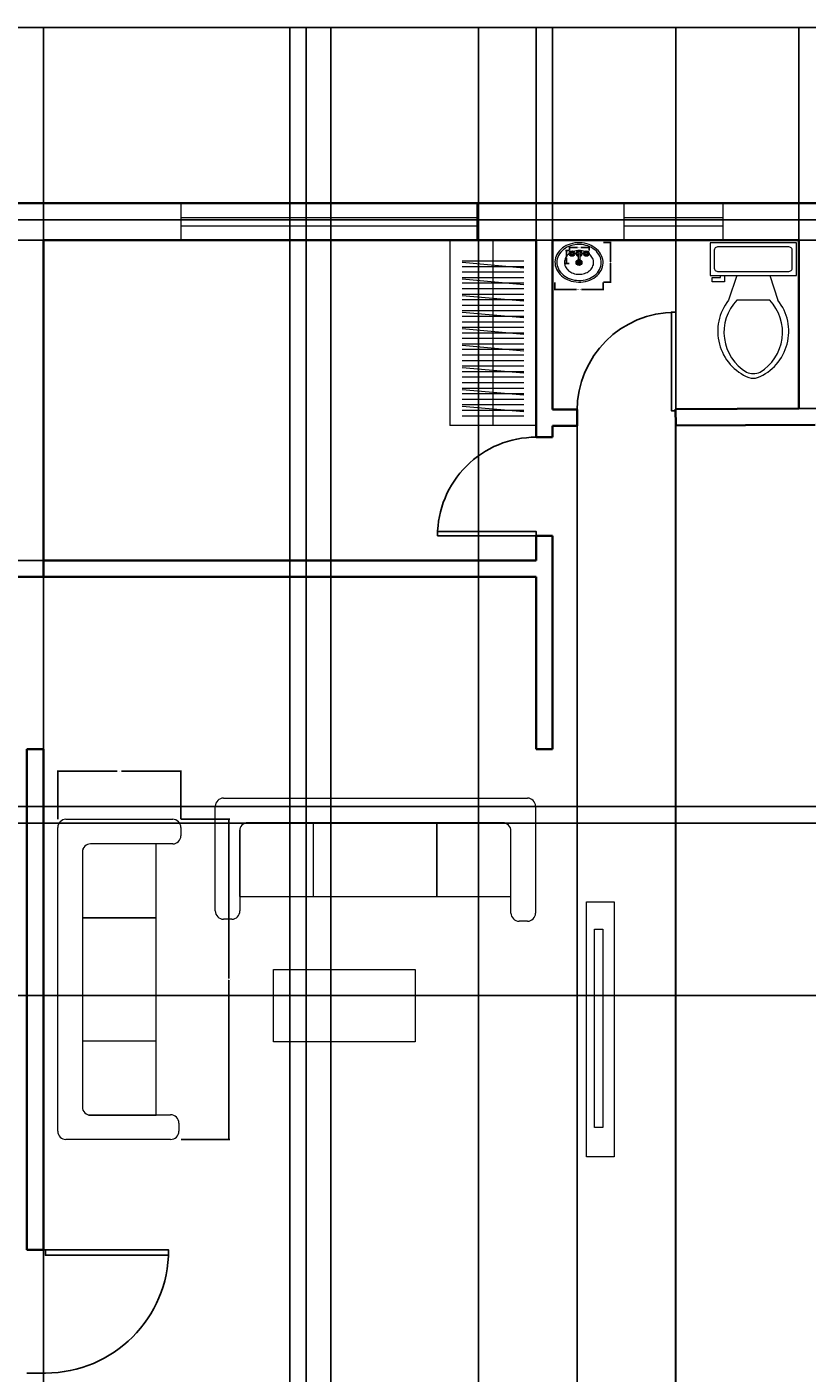
# Model space of a CAD drawing. Units: inches. Extents: x 2024 to 2965, y 1692 to 2308.
# Tile 6 of 8: x 2355 to 2545, y 1980 to 2308. Entities that reach past the tile are written whole.
import ezdxf

# ---------------------------------------------------------------- set-up
doc = ezdxf.new("R2010")
doc.units = ezdxf.units.IN
for name, color, linetype, lineweight in [('A-ANNO-DIMS', 2, 'Continuous', 18), ('A-DOOR', 3, 'Continuous', 25), ('A-EQPM', 6, 'Continuous', 18), ('A-FLOR-CASE', 33, 'Continuous', 20), ('A-FLOR-CASE-PATT', 252, 'Continuous', 13), ('A-FLOR-FIXT', 9, 'Continuous', 18), ('A-FURN', 8, 'Continuous', 18), ('A-GLAZ', 4, 'Continuous', 18), ('A-WALL', 7, 'Continuous', 35)]:
    doc.layers.add(name, color=color, linetype=linetype, lineweight=lineweight)
doc.styles.get("Standard").update_dxf_attribs({"font": 'arial.ttf'})
doc.dimstyles.get("Standard").update_dxf_attribs({"dimtxt": 0.18, "dimasz": 0.18, "dimexe": 0.18, "dimexo": 0.0625, "dimgap": 0.09, "dimtad": 0, "dimtih": 1, "dimtoh": 1, "dimdec": 4, "dimzin": 0, "dimdsep": 46, "dimtxsty": 'Standard', "dimcen": 0.09, "dimadec": 0, "dimazin": 0, "dimtfac": 1, "dimtdec": 4, "dimtofl": 0, "dimtmove": 0, "dimatfit": 3, "dimfxl": 1, "dimtolj": 1, "dimtzin": 0, "dimarcsym": 0})

# ---------------------------------------------------------------- blocks, each defined once
blk = doc.blocks.new('*U7')
for p, q in [((0, 0), (0, -6)), ((40, 0), (40, -6))]:
    blk.add_line(p, q)
blk.add_lwpolyline([(0, 0), (0, 40), (1.75, 40), (1.75, 0)], close=True)
blk.add_arc((0, 0), 40, 0, 90)
blk = doc.blocks.new('*U6')
for p, q in [((0, 0), (0, 6)), ((40, 0), (40, 6))]:
    blk.add_line(p, q)
blk.add_lwpolyline([(0, 0), (0, -40), (1.75, -40), (1.75, 0)], close=True)
blk.add_arc((0, 0), 40, 270, 0)
blk = doc.blocks.new('Sink - Oval top')
for p, q in [((-1, 0), (1, 0)), ((0, 1), (0, -1))]:
    blk.add_line(p, q)
for points in [[(-12.23, 0.39, 0.117634), (-11.46, -3.36, 0.104469), (-8.88, -6.8, 0.090016), (-5.08, -9.07, 0.08192), (-0.32, -10.02, 0.08192), (4.49, -9.38, 0.090016), (8.42, -7.36, 0.104469), (11.22, -4.09, 0.117634), (12.23, -0.39, 0.117634), (11.46, 3.36, 0.104469), (8.88, 6.8, 0.090016), (5.08, 9.07, 0.08192), (0.32, 10.02, 0.08192), (-4.49, 9.38, 0.090016), (-8.42, 7.36, 0.104469), (-11.22, 4.09, 0.117634)], [(-11.29, 0.16, 0.118622), (-10.52, -3.25, 0.104678), (-8.07, -6.36, 0.089562), (-4.54, -8.37, 0.081185), (-0.13, -9.15, 0.081185), (4.3, -8.49, 0.089562), (7.89, -6.58, 0.104678), (10.42, -3.55, 0.118622), (11.29, -0.16, 0.118622), (10.52, 3.25, 0.104678), (8.07, 6.36, 0.089562), (4.54, 8.37, 0.081185), (0.13, 9.15, 0.081185), (-4.3, 8.49, 0.089562), (-7.89, 6.58, 0.104678), (-10.42, 3.55, 0.118622)], [(-7.42, 0.08, 0.118283), (-6.91, -2.17, 0.104607), (-5.29, -4.21, 0.089718), (-2.97, -5.53, 0.081436), (-0.07, -6.04, 0.081436), (2.84, -5.59, 0.089718), (5.2, -4.33, 0.104607), (6.86, -2.32, 0.118283), (7.42, -0.08, 0.118283), (6.91, 2.17, 0.104607), (5.29, 4.21, 0.089718), (2.97, 5.53, 0.081436), (0.07, 6.04, 0.081436), (-2.84, 5.59, 0.089718), (-5.2, 4.33, 0.104607), (-6.86, 2.32, 0.118283)]]:
    blk.add_lwpolyline(points, format="xyb", close=True)
for radius in [1.5, 1]:
    blk.add_circle((0, 0), radius)
blk = doc.blocks.new('Faucet - Bathroom top')
for p, q in [((-4.107, 0.125), (-4.375, 0.125)), ((-3.75, 0.4788), (-3.75, 0.75)), ((-3.5, 0.482), (-3.5, 0.75)), ((-3.1461, 0.125), (-2.875, 0.125)), ((3.143, 0.125), (2.875, 0.125)), ((3.5, 0.4788), (3.5, 0.75)), ((3.75, 0.482), (3.75, 0.75)), ((4.1039, 0.125), (4.375, 0.125)), ((-4.1039, -0.125), (-4.375, -0.125)), ((-3.75, -0.4821), (-3.75, -0.75)), ((-3.5, -0.4789), (-3.5, -0.75)), ((-3.143, -0.125), (-2.875, -0.125)), ((-0.5, -0.8639), (-0.5, -4.5)), ((0.5, -4.5), (0.5, -0.8631)), ((3.1461, -0.125), (2.875, -0.125)), ((3.5, -0.4821), (3.5, -0.75)), ((3.75, -0.4789), (3.75, -0.75)), ((4.107, -0.125), (4.375, -0.125))]:
    blk.add_line(p, q)
for centre, radius in [((-3.625, 0), 1.375), ((-4.625, 0), 0.2795), ((-3.625, 0), 0.5), ((-3.625, 1), 0.2795), ((-2.625, 0), 0.2795), ((0, 0), 0.5), ((3.625, 0), 1.375), ((2.625, 0), 0.2795), ((3.625, 0), 0.5), ((3.625, 1), 0.2795), ((4.625, 0), 0.2795), ((-3.625, -1), 0.2795), ((3.625, -1), 0.2795)]:
    blk.add_circle(centre, radius)
for centre, radius, start, end in [((-3.625, 0), 1, 105.2407, 164.2093), ((-3.625, 0), 1, 16.44125, 74.07887), ((0, 0), 1.5, 289.6514, 250.3603), ((0, 0), 1, 300.3431, 239.7554), ((3.625, 0), 1, 106.12, 164.0884), ((3.625, 0), 1, 16.23422, 73.90469), ((-3.625, 0), 1, 196.2342, 253.9047), ((-3.625, 0), 1, 286.12, 344.0884), ((0, -4.5), 0.5, 180, 0), ((3.625, 0), 1, 196.4413, 254.0789), ((3.625, 0), 1, 285.2407, 344.2093)]:
    blk.add_arc(centre, radius, start, end)
blk = doc.blocks.new('Toilet - top')
for p, q in [((9.5, -6), (9.5, -2)), ((-10, -8.5), (-8, -8.5)), ((-10, -9.5), (-10, -8.5)), ((-7, -9.5), (-10, -9.5)), ((-8, -8.5), (-8, -8)), ((-7, -8), (-7, -9.5)), ((-4, -8), (-6, -14)), ((4, -8), (6, -14)), ((4, -14), (-4, -14))]:
    blk.add_line(p, q)
blk.add_lwpolyline([(10.5, -8), (10.5, 0), (-10.5, 0), (-10.5, -8)], close=True)
for points in [[(-9.5, -2), (-9.5, -6)], [(8.5, -1), (-8.5, -1)], [(-8.5, -7), (8.5, -7)]]:
    blk.add_lwpolyline(points)
for centre, radius, start, end in [((-8.62, -1.88), 0.884, 81.8699, 188.1301), ((8.62, -1.88), 0.884, 351.8699, 98.1301), ((-8.62, -6.12), 0.884, 171.8699, 278.1301), ((8.62, -6.12), 0.884, 261.8699, 8.1301), ((3.52, -21.58), 12.17, 141.4691, 247.9714), ((4.2, -21.82), 11.33, 136.3677, 238.9468), ((-3.52, -21.58), 12.17, 292.0284, 38.5307), ((-4.2, -21.82), 11.33, 301.053, 43.6321), ((0, -27.88), 4, 245.7318, 294.2682), ((0, -29), 4, 254.8605, 285.1395)]:
    blk.add_arc(centre, radius, start, end)
blk = doc.blocks.new('WIN-24-D9')
for p, q in [((0, 5.5), (24, 5.5)), ((0, 3.5), (24, 3.5))]:
    blk.add_line(p, q)
for points in [[(0, 0), (0, 9)], [(24, 9), (24, 0)]]:
    blk.add_lwpolyline(points)
blk = doc.blocks.new('WIN-72-D9')
for p, q in [((0, 5.5), (72, 5.5)), ((0, 3.5), (72, 3.5))]:
    blk.add_line(p, q)
for points in [[(0, 0), (0, 9)], [(72, 9), (72, 0)]]:
    blk.add_lwpolyline(points)
blk = doc.blocks.new('SOFA-78')
for p, q in [((2, 30), (76, 30)), ((0, 2.5), (0, 28)), ((78, 28), (78, 2)), ((70, 24), (7.91, 24)), ((6, 22.6), (6, 2.5)), ((72, 2), (72, 22)), ((4, 0.5), (2, 0.5)), ((76, 0), (74, 0))]:
    blk.add_line(p, q)
for points in [[(23.94, 24), (7.91, 24, 0.414214), (5.91, 22), (5.91, 6.04), (23.94, 6.04)], [(70, 24), (53.97, 24), (53.97, 6.04), (72, 6.04), (72, 22, 0.414214)]]:
    blk.add_lwpolyline(points, format="xyb", close=True)
for points in [[(35.94, 24), (17.9, 24)], [(35.94, 6.04), (53.97, 6.04), (53.97, 24), (35.94, 24)], [(17.9, 6.04), (35.94, 6.04)]]:
    blk.add_lwpolyline(points)
for centre, start, end in [((2, 28), 90, 180), ((76, 28), 0, 90), ((70, 22), 0, 90), ((2, 2.5), 180, 270), ((4, 2.5), 270, 0), ((74, 2), 180, 270), ((76, 2), 270, 0)]:
    blk.add_arc(centre, 2, start, end)
blk = doc.blocks.new('COFFEE-TABLE')
blk.add_lwpolyline([(0, 17.56), (34.53, 17.56), (34.53, 0), (0, 0)], close=True)
blk = doc.blocks.new('*D39')
at = {"layer": 'A-ANNO-DIMS', "color": 0, "lineweight": -2, "transparency": 16777216}
for p, q in [((2392.47, 2114.69), (2404.29, 2114.69)), ((2404.11, 2114.51), (2404.11, 2075.87)), ((2404.11, 2036.87), (2404.11, 2075.5)), ((2392.47, 2036.69), (2404.29, 2036.69))]:
    blk.add_line(p, q, dxfattribs=at)
at = {"layer": 'A-ANNO-DIMS', "color": 0, "transparency": 16777216}
for points in [[(2404.08, 2114.51), (2404.14, 2114.51), (2404.11, 2114.69)], [(2404.08, 2036.87), (2404.14, 2036.87), (2404.11, 2036.69)]]:
    blk.add_solid(points, dxfattribs=at)
at = {"layer": 'Defpoints', "color": 0, "transparency": 16777216}
for p in [(2392.41, 2114.69), (2404.11, 2114.69), (2392.41, 2036.69)]:
    blk.add_point(p, dxfattribs=at)
at = {"layer": 'A-ANNO-DIMS', "color": 0, "transparency": 16777216, "insert": (2404.11, 2075.69), "char_height": 0.18, "attachment_point": 5}
blk.add_mtext('\\A1;SOFA 78 TYP.', dxfattribs=at)
blk = doc.blocks.new('*D40')
at = {"layer": 'A-ANNO-DIMS', "color": 0, "lineweight": -2, "transparency": 16777216}
for p, q in [((2362.41, 2114.75), (2362.41, 2126.57)), ((2362.59, 2126.39), (2376.88, 2126.39)), ((2392.23, 2126.39), (2377.93, 2126.39)), ((2392.41, 2114.75), (2392.41, 2126.57))]:
    blk.add_line(p, q, dxfattribs=at)
at = {"layer": 'A-ANNO-DIMS', "color": 0, "transparency": 16777216}
for points in [[(2362.59, 2126.42), (2362.59, 2126.36), (2362.41, 2126.39)], [(2392.23, 2126.42), (2392.23, 2126.36), (2392.41, 2126.39)]]:
    blk.add_solid(points, dxfattribs=at)
at = {"layer": 'Defpoints', "color": 0, "transparency": 16777216}
for p in [(2362.41, 2126.39), (2362.41, 2114.69), (2392.41, 2114.69)]:
    blk.add_point(p, dxfattribs=at)
at = {"layer": 'A-ANNO-DIMS', "color": 0, "transparency": 16777216, "insert": (2377.41, 2126.39), "char_height": 0.18, "attachment_point": 5}
blk.add_mtext('\\A1;30 TYP.', dxfattribs=at)
blk = doc.blocks.new('*D61')
at = {"layer": 'A-ANNO-DIMS', "color": 0, "lineweight": -2, "transparency": 16777216}
for p, q in [((2483.49, 2245.46), (2483.49, 2243.58)), ((2483.67, 2243.76), (2488.74, 2243.76)), ((2495.07, 2243.76), (2490, 2243.76)), ((2495.25, 2245.46), (2495.25, 2243.58))]:
    blk.add_line(p, q, dxfattribs=at)
at = {"layer": 'A-ANNO-DIMS', "color": 0, "transparency": 16777216}
for points in [[(2483.67, 2243.79), (2483.67, 2243.73), (2483.49, 2243.76)], [(2495.07, 2243.79), (2495.07, 2243.73), (2495.25, 2243.76)]]:
    blk.add_solid(points, dxfattribs=at)
at = {"layer": 'Defpoints', "color": 0, "transparency": 16777216}
for p in [(2483.49, 2245.52), (2495.25, 2245.52), (2495.25, 2243.76)]:
    blk.add_point(p, dxfattribs=at)
at = {"layer": 'A-ANNO-DIMS', "color": 0, "transparency": 16777216, "insert": (2489.37, 2243.76), "char_height": 0.18, "attachment_point": 5}
blk.add_mtext('\\A1;BASIN 12', dxfattribs=at)
blk = doc.blocks.new('*D62')
at = {"layer": 'A-ANNO-DIMS', "color": 0, "lineweight": -2, "transparency": 16777216}
for p, q in [((2495.31, 2255.17), (2497.19, 2255.17)), ((2497.01, 2254.99), (2497.01, 2250.53)), ((2497.01, 2245.7), (2497.01, 2250.17)), ((2495.31, 2245.52), (2497.19, 2245.52))]:
    blk.add_line(p, q, dxfattribs=at)
at = {"layer": 'A-ANNO-DIMS', "color": 0, "transparency": 16777216}
for points in [[(2496.98, 2254.99), (2497.04, 2254.99), (2497.01, 2255.17)], [(2496.98, 2245.7), (2497.04, 2245.7), (2497.01, 2245.52)]]:
    blk.add_solid(points, dxfattribs=at)
at = {"layer": 'Defpoints', "color": 0, "transparency": 16777216}
for p in [(2495.25, 2255.17), (2497.01, 2255.17), (2495.25, 2245.52)]:
    blk.add_point(p, dxfattribs=at)
at = {"layer": 'A-ANNO-DIMS', "color": 0, "transparency": 16777216, "insert": (2497.01, 2250.35), "char_height": 0.18, "attachment_point": 5}
blk.add_mtext('\\A1;10', dxfattribs=at)
blk = doc.blocks.new('*D67')
at = {"layer": 'A-ANNO-DIMS', "color": 0, "lineweight": -2, "transparency": 16777216}
for p, q in [((2487.01, 2253.3), (2487.01, 2254.14)), ((2487.19, 2253.96), (2488.97, 2253.96)), ((2491.62, 2253.96), (2489.83, 2253.96)), ((2491.8, 2253.3), (2491.8, 2254.14))]:
    blk.add_line(p, q, dxfattribs=at)
at = {"layer": 'A-ANNO-DIMS', "color": 0, "transparency": 16777216}
for points in [[(2487.19, 2253.99), (2487.19, 2253.93), (2487.01, 2253.96)], [(2491.62, 2253.99), (2491.62, 2253.93), (2491.8, 2253.96)]]:
    blk.add_solid(points, dxfattribs=at)
at = {"layer": 'Defpoints', "color": 0, "transparency": 16777216}
for p in [(2487.01, 2253.24), (2491.8, 2253.96), (2491.8, 2253.24)]:
    blk.add_point(p, dxfattribs=at)
at = {"layer": 'A-ANNO-DIMS', "color": 0, "transparency": 16777216, "insert": (2489.4, 2253.96), "char_height": 0.18, "attachment_point": 5}
blk.add_mtext('\\A1;TAP 5', dxfattribs=at)
blk = doc.blocks.new('*D68')
at = {"layer": 'A-ANNO-DIMS', "color": 0, "lineweight": -2, "transparency": 16777216}
for p, q in [((2486.94, 2253.24), (2486.11, 2253.24)), ((2486.29, 2253.06), (2486.29, 2251.86)), ((2486.94, 2250.13), (2486.11, 2250.13)), ((2486.29, 2250.31), (2486.29, 2251.5))]:
    blk.add_line(p, q, dxfattribs=at)
at = {"layer": 'A-ANNO-DIMS', "color": 0, "transparency": 16777216}
for points in [[(2486.26, 2253.06), (2486.32, 2253.06), (2486.29, 2253.24)], [(2486.26, 2250.31), (2486.32, 2250.31), (2486.29, 2250.13)]]:
    blk.add_solid(points, dxfattribs=at)
at = {"layer": 'Defpoints', "color": 0, "transparency": 16777216}
for p in [(2486.29, 2253.24), (2487.01, 2253.24), (2487.01, 2250.13)]:
    blk.add_point(p, dxfattribs=at)
at = {"layer": 'A-ANNO-DIMS', "color": 0, "transparency": 16777216, "insert": (2486.29, 2251.68), "char_height": 0.18, "attachment_point": 5}
blk.add_mtext('\\A1;3', dxfattribs=at)
blk = doc.blocks.new('*D76')
at = {"layer": 'A-ANNO-DIMS', "color": 0, "lineweight": -2, "transparency": 16777216}
for p, q in [((2718.97, 2264.77), (2964.97, 2264.77)), ((2964.79, 2264.59), (2964.79, 2000.12)), ((2964.79, 1735.28), (2964.79, 1999.75)), ((2515.28, 1735.1), (2964.97, 1735.1))]:
    blk.add_line(p, q, dxfattribs=at)
at = {"layer": 'A-ANNO-DIMS', "color": 0, "transparency": 16777216}
for points in [[(2964.76, 2264.59), (2964.82, 2264.59), (2964.79, 2264.77)], [(2964.76, 1735.28), (2964.82, 1735.28), (2964.79, 1735.1)]]:
    blk.add_solid(points, dxfattribs=at)
at = {"layer": 'Defpoints', "color": 0, "transparency": 16777216}
for p in [(2718.91, 2264.77), (2515.22, 1735.1), (2964.79, 1735.1)]:
    blk.add_point(p, dxfattribs=at)
at = {"layer": 'A-ANNO-DIMS', "color": 0, "transparency": 16777216, "insert": (2964.79, 1999.94), "char_height": 0.18, "attachment_point": 5}
blk.add_mtext('\\A1;529.7', dxfattribs=at)
blk = doc.blocks.new('*D80')
at = {"layer": 'A-ANNO-DIMS', "color": 0, "lineweight": -2, "transparency": 16777216}
for p, q in [((2358.91, 2255.84), (2358.91, 2307.73)), ((2359.09, 2307.55), (2418.63, 2307.55)), ((2478.73, 2307.55), (2419.19, 2307.55)), ((2478.91, 2255.84), (2478.91, 2307.73))]:
    blk.add_line(p, q, dxfattribs=at)
at = {"layer": 'A-ANNO-DIMS', "color": 0, "transparency": 16777216}
for points in [[(2359.09, 2307.58), (2359.09, 2307.52), (2358.91, 2307.55)], [(2478.73, 2307.58), (2478.73, 2307.52), (2478.91, 2307.55)]]:
    blk.add_solid(points, dxfattribs=at)
at = {"layer": 'Defpoints', "color": 0, "transparency": 16777216}
for p in [(2478.91, 2307.55), (2358.91, 2255.77), (2478.91, 2255.77)]:
    blk.add_point(p, dxfattribs=at)
at = {"layer": 'A-ANNO-DIMS', "color": 0, "transparency": 16777216, "insert": (2418.91, 2307.55), "char_height": 0.18, "attachment_point": 5}
blk.add_mtext('\\A1;120', dxfattribs=at)
blk = doc.blocks.new('*D81')
at = {"layer": 'A-ANNO-DIMS', "color": 0, "lineweight": -2, "transparency": 16777216}
for p, q in [((2478.84, 2255.77), (2024.5, 2255.77)), ((2024.68, 2255.59), (2024.68, 2216.96)), ((2024.68, 2177.95), (2024.68, 2216.59)), ((2478.84, 2177.77), (2024.5, 2177.77))]:
    blk.add_line(p, q, dxfattribs=at)
at = {"layer": 'A-ANNO-DIMS', "color": 0, "transparency": 16777216}
for points in [[(2024.65, 2255.59), (2024.71, 2255.59), (2024.68, 2255.77)], [(2024.65, 2177.95), (2024.71, 2177.95), (2024.68, 2177.77)]]:
    blk.add_solid(points, dxfattribs=at)
at = {"layer": 'Defpoints', "color": 0, "transparency": 16777216}
for p in [(2478.91, 2255.77), (2024.68, 2177.77), (2478.91, 2177.77)]:
    blk.add_point(p, dxfattribs=at)
at = {"layer": 'A-ANNO-DIMS', "color": 0, "transparency": 16777216, "insert": (2024.68, 2216.77), "char_height": 0.18, "attachment_point": 5}
blk.add_mtext('\\A1;78', dxfattribs=at)
blk = doc.blocks.new('*D84')
at = {"layer": 'A-ANNO-DIMS', "color": 0, "lineweight": -2, "transparency": 16777216}
for p, q in [((2618.84, 2255.77), (2024.5, 2255.77)), ((2024.68, 2255.59), (2024.68, 2163.96)), ((2024.68, 2071.95), (2024.68, 2163.59)), ((2618.84, 2071.77), (2024.5, 2071.77))]:
    blk.add_line(p, q, dxfattribs=at)
at = {"layer": 'A-ANNO-DIMS', "color": 0, "transparency": 16777216}
for points in [[(2024.65, 2255.59), (2024.71, 2255.59), (2024.68, 2255.77)], [(2024.65, 2071.95), (2024.71, 2071.95), (2024.68, 2071.77)]]:
    blk.add_solid(points, dxfattribs=at)
at = {"layer": 'Defpoints', "color": 0, "transparency": 16777216}
for p in [(2024.68, 2255.77), (2618.91, 2255.77), (2618.91, 2071.77)]:
    blk.add_point(p, dxfattribs=at)
at = {"layer": 'A-ANNO-DIMS', "color": 0, "transparency": 16777216, "insert": (2024.68, 2163.77), "char_height": 0.18, "attachment_point": 5}
blk.add_mtext('\\A1;184', dxfattribs=at)
blk = doc.blocks.new('*D88')
at = {"layer": 'A-ANNO-DIMS', "color": 0, "lineweight": -2, "transparency": 16777216}
for p, q in [((2817.84, 2260.77), (2024.5, 2260.77)), ((2024.68, 2260.59), (2024.68, 2189.46)), ((2024.68, 2117.95), (2024.68, 2189.09)), ((2817.84, 2117.77), (2024.5, 2117.77))]:
    blk.add_line(p, q, dxfattribs=at)
at = {"layer": 'A-ANNO-DIMS', "color": 0, "transparency": 16777216}
for points in [[(2024.65, 2260.59), (2024.71, 2260.59), (2024.68, 2260.77)], [(2024.65, 2117.95), (2024.71, 2117.95), (2024.68, 2117.77)]]:
    blk.add_solid(points, dxfattribs=at)
at = {"layer": 'Defpoints', "color": 0, "transparency": 16777216}
for p in [(2817.91, 2260.77), (2024.68, 2117.77), (2817.91, 2117.77)]:
    blk.add_point(p, dxfattribs=at)
at = {"layer": 'A-ANNO-DIMS', "color": 0, "transparency": 16777216, "insert": (2024.68, 2189.27), "char_height": 0.18, "attachment_point": 5}
blk.add_mtext('\\A1;143', dxfattribs=at)
blk = doc.blocks.new('*D93')
at = {"layer": 'A-ANNO-DIMS', "color": 0, "lineweight": -2, "transparency": 16777216}
for p, q in [((2187.46, 1932.41), (2187.46, 2307.73)), ((2187.64, 2307.55), (2302.72, 2307.55)), ((2418.73, 2307.55), (2303.65, 2307.55)), ((2418.91, 1933.84), (2418.91, 2307.73))]:
    blk.add_line(p, q, dxfattribs=at)
at = {"layer": 'A-ANNO-DIMS', "color": 0, "transparency": 16777216}
for points in [[(2187.64, 2307.58), (2187.64, 2307.52), (2187.46, 2307.55)], [(2418.73, 2307.58), (2418.73, 2307.52), (2418.91, 2307.55)]]:
    blk.add_solid(points, dxfattribs=at)
at = {"layer": 'Defpoints', "color": 0, "transparency": 16777216}
for p in [(2418.91, 2307.55), (2187.46, 1932.35), (2418.91, 1933.77)]:
    blk.add_point(p, dxfattribs=at)
at = {"layer": 'A-ANNO-DIMS', "color": 0, "transparency": 16777216, "insert": (2303.18, 2307.55), "char_height": 0.18, "attachment_point": 5}
blk.add_mtext('\\A1;231.45', dxfattribs=at)
blk = doc.blocks.new('*D96')
at = {"layer": 'A-ANNO-DIMS', "color": 0, "lineweight": -2, "transparency": 16777216}
for p, q in [((2358.91, 1889.84), (2358.91, 2307.73)), ((2359.09, 2307.55), (2388.69, 2307.55)), ((2418.73, 2307.55), (2389.13, 2307.55)), ((2418.91, 1889.84), (2418.91, 2307.73))]:
    blk.add_line(p, q, dxfattribs=at)
at = {"layer": 'A-ANNO-DIMS', "color": 0, "transparency": 16777216}
for points in [[(2359.09, 2307.58), (2359.09, 2307.52), (2358.91, 2307.55)], [(2418.73, 2307.58), (2418.73, 2307.52), (2418.91, 2307.55)]]:
    blk.add_solid(points, dxfattribs=at)
at = {"layer": 'Defpoints', "color": 0, "transparency": 16777216}
for p in [(2418.91, 2307.55), (2358.91, 1889.77), (2418.91, 1889.77)]:
    blk.add_point(p, dxfattribs=at)
at = {"layer": 'A-ANNO-DIMS', "color": 0, "transparency": 16777216, "insert": (2388.91, 2307.55), "char_height": 0.18, "attachment_point": 5}
blk.add_mtext('\\A1;60', dxfattribs=at)
blk = doc.blocks.new('*D98')
at = {"layer": 'A-ANNO-DIMS', "color": 0, "lineweight": -2, "transparency": 16777216}
for p, q in [((2422.91, 1973.84), (2422.91, 2307.73)), ((2423.09, 2307.55), (2543.62, 2307.55)), ((2664.73, 2307.55), (2544.2, 2307.55)), ((2664.91, 1956.85), (2664.91, 2307.73))]:
    blk.add_line(p, q, dxfattribs=at)
at = {"layer": 'A-ANNO-DIMS', "color": 0, "transparency": 16777216}
for points in [[(2423.09, 2307.58), (2423.09, 2307.52), (2422.91, 2307.55)], [(2664.73, 2307.58), (2664.73, 2307.52), (2664.91, 2307.55)]]:
    blk.add_solid(points, dxfattribs=at)
at = {"layer": 'Defpoints', "color": 0, "transparency": 16777216}
for p in [(2664.91, 2307.55), (2422.91, 1973.77), (2664.91, 1956.79)]:
    blk.add_point(p, dxfattribs=at)
at = {"layer": 'A-ANNO-DIMS', "color": 0, "transparency": 16777216, "insert": (2543.91, 2307.55), "char_height": 0.18, "attachment_point": 5}
blk.add_mtext('\\A1;242', dxfattribs=at)
blk = doc.blocks.new('*D101')
at = {"layer": 'A-ANNO-DIMS', "color": 0, "lineweight": -2, "transparency": 16777216}
for p, q in [((2917.96, 2113.77), (2024.5, 2113.77)), ((2024.68, 2113.59), (2024.68, 2035.52)), ((2024.68, 1957.09), (2024.68, 2035.16)), ((2917.96, 1956.91), (2024.5, 1956.91))]:
    blk.add_line(p, q, dxfattribs=at)
at = {"layer": 'A-ANNO-DIMS', "color": 0, "transparency": 16777216}
for points in [[(2024.65, 2113.59), (2024.71, 2113.59), (2024.68, 2113.77)], [(2024.65, 1957.09), (2024.71, 1957.09), (2024.68, 1956.91)]]:
    blk.add_solid(points, dxfattribs=at)
at = {"layer": 'Defpoints', "color": 0, "transparency": 16777216}
for p in [(2024.68, 2113.77), (2918.02, 2113.77), (2918.02, 1956.91)]:
    blk.add_point(p, dxfattribs=at)
at = {"layer": 'A-ANNO-DIMS', "color": 0, "transparency": 16777216, "insert": (2024.68, 2035.34), "char_height": 0.18, "attachment_point": 5}
blk.add_mtext('\\A1;156.87', dxfattribs=at)
blk = doc.blocks.new('*D103')
at = {"layer": 'A-ANNO-DIMS', "color": 0, "lineweight": -2, "transparency": 16777216}
for p, q in [((2464.91, 1881.44), (2464.91, 2307.73)), ((2465.09, 2307.55), (2488.68, 2307.55)), ((2512.73, 2307.55), (2489.13, 2307.55)), ((2512.91, 1881.44), (2512.91, 2307.73))]:
    blk.add_line(p, q, dxfattribs=at)
at = {"layer": 'A-ANNO-DIMS', "color": 0, "transparency": 16777216}
for points in [[(2465.09, 2307.58), (2465.09, 2307.52), (2464.91, 2307.55)], [(2512.73, 2307.58), (2512.73, 2307.52), (2512.91, 2307.55)]]:
    blk.add_solid(points, dxfattribs=at)
at = {"layer": 'Defpoints', "color": 0, "transparency": 16777216}
for p in [(2512.91, 2307.55), (2464.91, 1881.37), (2512.91, 1881.37)]:
    blk.add_point(p, dxfattribs=at)
at = {"layer": 'A-ANNO-DIMS', "color": 0, "transparency": 16777216, "insert": (2488.91, 2307.55), "char_height": 0.18, "attachment_point": 5}
blk.add_mtext('\\A1;48', dxfattribs=at)
blk = doc.blocks.new('*D107')
at = {"layer": 'A-ANNO-DIMS', "color": 0, "lineweight": -2, "transparency": 16777216}
for p, q in [((2482.91, 2255.84), (2482.91, 2307.73)), ((2483.09, 2307.55), (2512.69, 2307.55)), ((2542.73, 2307.55), (2513.13, 2307.55)), ((2542.91, 2255.84), (2542.91, 2307.73))]:
    blk.add_line(p, q, dxfattribs=at)
at = {"layer": 'A-ANNO-DIMS', "color": 0, "transparency": 16777216}
for points in [[(2483.09, 2307.58), (2483.09, 2307.52), (2482.91, 2307.55)], [(2542.73, 2307.58), (2542.73, 2307.52), (2542.91, 2307.55)]]:
    blk.add_solid(points, dxfattribs=at)
at = {"layer": 'Defpoints', "color": 0, "transparency": 16777216}
for p in [(2542.91, 2307.55), (2482.91, 2255.77), (2542.91, 2255.77)]:
    blk.add_point(p, dxfattribs=at)
at = {"layer": 'A-ANNO-DIMS', "color": 0, "transparency": 16777216, "insert": (2512.91, 2307.55), "char_height": 0.18, "attachment_point": 5}
blk.add_mtext('\\A1;60', dxfattribs=at)
blk = doc.blocks.new('*D108')
at = {"layer": 'A-ANNO-DIMS', "color": 0, "lineweight": -2, "transparency": 16777216}
for p, q in [((2542.97, 2255.77), (2964.97, 2255.77)), ((2964.79, 2255.59), (2964.79, 2235.45)), ((2964.79, 2214.95), (2964.79, 2235.09)), ((2542.97, 2214.77), (2964.97, 2214.77))]:
    blk.add_line(p, q, dxfattribs=at)
at = {"layer": 'A-ANNO-DIMS', "color": 0, "transparency": 16777216}
for points in [[(2964.76, 2255.59), (2964.82, 2255.59), (2964.79, 2255.77)], [(2964.76, 2214.95), (2964.82, 2214.95), (2964.79, 2214.77)]]:
    blk.add_solid(points, dxfattribs=at)
at = {"layer": 'Defpoints', "color": 0, "transparency": 16777216}
for p in [(2542.91, 2255.77), (2542.91, 2214.77), (2964.79, 2214.77)]:
    blk.add_point(p, dxfattribs=at)
at = {"layer": 'A-ANNO-DIMS', "color": 0, "transparency": 16777216, "insert": (2964.79, 2235.27), "char_height": 0.18, "attachment_point": 5}
blk.add_mtext('\\A1;41', dxfattribs=at)
blk = doc.blocks.new('*D109')
at = {"layer": 'A-ANNO-DIMS', "color": 0, "lineweight": -2, "transparency": 16777216}
for p, q in [((2488.89, 2214.47), (2488.89, 1692.14)), ((2512.89, 2214.58), (2512.89, 1692.14)), ((2489.07, 1692.32), (2500.67, 1692.32)), ((2512.71, 1692.32), (2501.11, 1692.32))]:
    blk.add_line(p, q, dxfattribs=at)
at = {"layer": 'A-ANNO-DIMS', "color": 0, "transparency": 16777216}
for points in [[(2489.07, 1692.35), (2489.07, 1692.29), (2488.89, 1692.32)], [(2512.71, 1692.35), (2512.71, 1692.29), (2512.89, 1692.32)]]:
    blk.add_solid(points, dxfattribs=at)
at = {"layer": 'Defpoints', "color": 0, "transparency": 16777216}
for p in [(2488.89, 2214.53), (2512.89, 2214.64), (2512.89, 1692.32)]:
    blk.add_point(p, dxfattribs=at)
at = {"layer": 'A-ANNO-DIMS', "color": 0, "transparency": 16777216, "insert": (2500.89, 1692.32), "char_height": 0.18, "attachment_point": 5}
blk.add_mtext('\\A1;24', dxfattribs=at)
blk = doc.blocks.new('*D114')
at = {"layer": 'A-ANNO-DIMS', "color": 0, "lineweight": -2, "transparency": 16777216}
for p, q in [((2428.91, 1761.01), (2428.91, 2307.73)), ((2429.09, 2307.55), (2488.63, 2307.55)), ((2548.73, 2307.55), (2489.19, 2307.55)), ((2548.91, 1761.01), (2548.91, 2307.73))]:
    blk.add_line(p, q, dxfattribs=at)
at = {"layer": 'A-ANNO-DIMS', "color": 0, "transparency": 16777216}
for points in [[(2429.09, 2307.58), (2429.09, 2307.52), (2428.91, 2307.55)], [(2548.73, 2307.58), (2548.73, 2307.52), (2548.91, 2307.55)]]:
    blk.add_solid(points, dxfattribs=at)
at = {"layer": 'Defpoints', "color": 0, "transparency": 16777216}
for p in [(2548.91, 2307.55), (2428.91, 1760.95), (2548.91, 1760.95)]:
    blk.add_point(p, dxfattribs=at)
at = {"layer": 'A-ANNO-DIMS', "color": 0, "transparency": 16777216, "insert": (2488.91, 2307.55), "char_height": 0.18, "attachment_point": 5}
blk.add_mtext('\\A1;120', dxfattribs=at)

msp = doc.modelspace()

# ---------------------------------------------------------------- hatches: boundary and pattern name
at = {"layer": 'A-FLOR-CASE-PATT'}
h = msp.add_hatch(dxfattribs=at)
h.set_pattern_fill('ANSI31', color=256, scale=0.4242327, angle=-45, style=0)
h.paths.add_polyline_path([(2460.9061, 2212.6716), (2475.9061, 2212.6716), (2475.9061, 2251.7328), (2460.9061, 2251.7328)])

# ---------------------------------------------------------------- linework, layer by layer
at = {"layer": 'A-EQPM'}
for points in [[(2491.2012, 2094.5874), (2497.9618, 2094.5874), (2497.9618, 2032.4829), (2491.2012, 2032.4829)], [(2493.0963, 2087.9089), (2495.1918, 2087.9089), (2495.1918, 2039.6365), (2493.0963, 2039.6365)]]:
    msp.add_lwpolyline(points, close=True, dxfattribs=at)
at = {"layer": 'A-FLOR-CASE'}
for p, q in [((2478.9061, 2255.7736), (2457.9061, 2255.7736)), ((2457.9061, 2255.7736), (2457.9061, 2210.6511)), ((2468.4061, 2255.7736), (2468.4061, 2210.6511)), ((2478.9061, 2210.6511), (2478.9061, 2255.7736)), ((2478.9061, 2210.6511), (2457.9061, 2210.6511))]:
    msp.add_line(p, q, dxfattribs=at)
at = {"layer": 'A-FLOR-CASE-PATT'}
for p, q in [((2460.9061, 2250.3858), (2475.9061, 2249.0389)), ((2460.9061, 2246.345), (2475.9061, 2244.9981)), ((2460.9061, 2242.3042), (2475.9061, 2240.9573)), ((2460.9061, 2238.2634), (2475.9061, 2236.9164)), ((2460.9061, 2234.2226), (2475.9061, 2232.8756)), ((2460.9061, 2230.1818), (2475.9061, 2228.8348)), ((2460.9061, 2224.794), (2475.9061, 2223.4471)), ((2460.9061, 2219.4062), (2475.9061, 2218.0593)), ((2460.9061, 2215.3654), (2475.9061, 2214.0185))]:
    msp.add_line(p, q, dxfattribs=at)
at = {"layer": 'A-WALL'}
for p, q in [((2161.9061, 2264.7736), (2821.9061, 2264.7736)), ((2358.9061, 2255.7736), (2478.9061, 2255.7736)), ((2358.9061, 2173.7736), (2358.9061, 2255.7736)), ((2478.9061, 2207.7736), (2478.9061, 2255.7736)), ((2482.9061, 2255.7736), (2542.9061, 2255.7736)), ((2482.9061, 2214.5068), (2482.9061, 2255.7736)), ((2542.9061, 2214.7696), (2542.9061, 2255.7736)), ((2482.8886, 2214.5067), (2488.8886, 2214.533)), ((2488.9061, 2210.5331), (2488.8886, 2214.533)), ((2512.8883, 2214.6382), (2542.9061, 2214.7696)), ((2512.9058, 2210.6382), (2512.8883, 2214.6382)), ((2482.9061, 2210.5068), (2488.9061, 2210.5331)), ((2482.9061, 2207.7736), (2482.9061, 2210.5068)), ((2512.9058, 2210.6382), (2546.9061, 2210.7871)), ((2478.9061, 2207.7736), (2482.9061, 2207.7736)), ((2478.9061, 2177.7736), (2478.9061, 2183.7736)), ((2478.9061, 2183.7736), (2482.9061, 2183.7736)), ((2482.9061, 2131.7736), (2482.9061, 2183.7736)), ((2358.9061, 2177.7736), (2478.9061, 2177.7736)), ((2294.9061, 2173.7736), (2478.9061, 2173.7736)), ((2478.9061, 2131.7736), (2478.9061, 2173.7736)), ((2354.9061, 2131.7736), (2358.9061, 2131.7736)), ((2354.9061, 2009.7736), (2354.9061, 2131.7736)), ((2358.9061, 2009.7736), (2358.9061, 2131.7736)), ((2478.9061, 2131.7736), (2482.9061, 2131.7736)), ((2354.9061, 2009.7736), (2358.9061, 2009.7736))]:
    msp.add_line(p, q, dxfattribs=at)

# ---------------------------------------------------------------- block references
at = {"layer": 'A-DOOR', "xscale": -0.6, "yscale": 0.6, "zscale": 0.6}
msp.add_blockref('*U7', (2512.9058, 2214.2382), dxfattribs=at)
at = {"layer": 'A-DOOR', "rotation": 270}
for name, p, xscale, yscale, zscale in [('*U6', (2478.9061, 2183.7736), -0.6, 0.6, 0.6), ('*U7', (2359.4061, 2009.7736), 0.75, 0.75, 0.75)]:
    msp.add_blockref(name, p, dxfattribs=dict(at, xscale=xscale, yscale=yscale, zscale=zscale))
at = {"layer": 'A-FLOR-FIXT', "xscale": 0.4790267857601149, "yscale": 0.4790267857601149, "zscale": 0.4790267857601149}
for name, p in [('Sink - Oval top', (2489.3689, 2250.3474)), ('Faucet - Bathroom top', (2489.4014, 2252.5206))]:
    msp.add_blockref(name, p, dxfattribs=at)
at = {"layer": 'A-FLOR-FIXT'}
msp.add_blockref('Toilet - top', (2531.7998, 2255.145), dxfattribs=at)
at = {"layer": 'A-FURN'}
for name, p in [('SOFA-78', (2400.7895, 2089.852)), ('COFFEE-TABLE', (2414.959, 2060.4956))]:
    msp.add_blockref(name, p, dxfattribs=at)
at = {"layer": 'A-FURN', "rotation": 89.99960837471713}
msp.add_blockref('SOFA-78', (2392.4058, 2036.6882), dxfattribs=at)
at = {"layer": 'A-GLAZ'}
for name, p in [('WIN-72-D9', (2392.4783, 2255.774)), ('WIN-24-D9', (2500.3864, 2255.774))]:
    msp.add_blockref(name, p, dxfattribs=at)

# ---------------------------------------------------------------- dimensions: what is measured, and where the dimension line sits
at = {"layer": 'A-ANNO-DIMS'}
for base, p1, p2, override, picture, middle in [((2418.9061, 2307.5486), (2187.4594, 1932.352), (2418.9061, 1933.7736), {"dimdec": 2, "dimlfac": 1, "dimrnd": 0, "dimzin": 0, "dimdsep": 46, "dimlunit": 2}, '*D93', (2303.1828, 2307.5486)), ((2478.9061, 2307.5486), (2358.9061, 2255.7736), (2478.9061, 2255.7736), {"dimdec": 0, "dimlfac": 1, "dimrnd": 0, "dimzin": 0, "dimdsep": 46, "dimlunit": 2}, '*D80', (2418.9061, 2307.5486)), ((2418.9061, 2307.5486), (2358.9061, 1889.7736), (2418.9061, 1889.7736), {"dimdec": 0, "dimlfac": 1, "dimrnd": 0, "dimzin": 0, "dimdsep": 46, "dimlunit": 2}, '*D96', (2388.9061, 2307.5486)), ((2664.9061, 2307.5486), (2422.9061, 1973.7736), (2664.9061, 1956.7881), {"dimdec": 0, "dimlfac": 1, "dimrnd": 0, "dimzin": 0, "dimdsep": 46, "dimlunit": 2}, '*D98', (2543.9061, 2307.5486)), ((2548.9061, 2307.5486), (2428.9061, 1760.9504), (2548.9061, 1760.9504), {"dimdec": 0, "dimlfac": 1, "dimrnd": 0, "dimzin": 0, "dimdsep": 46, "dimlunit": 2}, '*D114', (2488.9061, 2307.5486)), ((2512.9061, 2307.5486), (2464.9061, 1881.3736), (2512.9061, 1881.3736), {"dimdec": 0, "dimlfac": 1, "dimrnd": 0, "dimzin": 0, "dimdsep": 46, "dimlunit": 2}, '*D103', (2488.9061, 2307.5486)), ((2542.9061, 2307.5486), (2482.9061, 2255.7736), (2542.9061, 2255.7736), {"dimdec": 0, "dimlfac": 1, "dimrnd": 0, "dimzin": 0, "dimdsep": 46, "dimlunit": 2}, '*D107', (2512.9061, 2307.5486)), ((2512.8883, 1692.3236), (2488.8886, 2214.533), (2512.8883, 2214.6382), {"dimdec": 0, "dimlfac": 1, "dimrnd": 0, "dimzin": 0, "dimdsep": 46, "dimlunit": 2}, '*D109', (2500.8884, 1692.3236))]:
    dim = msp.add_linear_dim(base=base, p1=p1, p2=p2, dimstyle='Standard', override=override, dxfattribs=at)
    dim.commit()
    dim.dimension.update_dxf_attribs({"geometry": picture, "text_midpoint": middle})
for base, p1, p2, override, picture, middle in [((2964.7942, 1735.0986), (2718.9061, 2264.7736), (2515.2195, 1735.0986), {"dimdec": 1, "dimlfac": 1, "dimrnd": 0, "dimzin": 0, "dimdsep": 46, "dimlunit": 2}, '*D76', (2964.7942, 1999.9361)), ((2024.6844, 2117.7736), (2817.9061, 2260.7736), (2817.9061, 2117.7736), {"dimdec": 0, "dimlfac": 1, "dimrnd": 0, "dimzin": 0, "dimdsep": 46, "dimlunit": 2}, '*D88', (2024.6844, 2189.2736)), ((2024.6844, 2255.7736), (2618.9061, 2071.7736), (2618.9061, 2255.7736), {"dimdec": 0, "dimlfac": 1, "dimrnd": 0, "dimzin": 0, "dimdsep": 46, "dimlunit": 2}, '*D84', (2024.6844, 2163.7736)), ((2024.6844, 2177.7736), (2478.9061, 2255.7736), (2478.9061, 2177.7736), {"dimdec": 0, "dimlfac": 1, "dimrnd": 0, "dimzin": 0, "dimdsep": 46, "dimlunit": 2}, '*D81', (2024.6844, 2216.7736)), ((2486.2877, 2253.2392), (2487.0062, 2250.1255), (2487.0062, 2253.2392), {"dimdec": 0, "dimlfac": 1, "dimrnd": 0, "dimzin": 0, "dimdsep": 46, "dimlunit": 2}, '*D68', (2486.2877, 2251.6823)), ((2497.0133, 2255.1703), (2495.2492, 2245.5244), (2495.2492, 2255.1703), {"dimdec": 0, "dimlfac": 1, "dimrnd": 0, "dimzin": 0, "dimdsep": 46, "dimlunit": 2}, '*D62', (2497.0133, 2250.3474)), ((2964.7942, 2214.7696), (2542.9061, 2255.7736), (2542.9061, 2214.7696), {"dimdec": 0, "dimlfac": 1, "dimrnd": 0, "dimzin": 0, "dimdsep": 46, "dimlunit": 2}, '*D108', (2964.7942, 2235.2716)), ((2024.6844, 2113.7736), (2918.0192, 1956.9082), (2918.0192, 2113.7736), {"dimdec": 2, "dimlfac": 1, "dimrnd": 0, "dimzin": 0, "dimdsep": 46, "dimlunit": 2}, '*D101', (2024.6844, 2035.3409))]:
    dim = msp.add_linear_dim(base=base, p1=p1, p2=p2, angle=90, dimstyle='Standard', override=override, dxfattribs=at)
    dim.commit()
    dim.dimension.update_dxf_attribs({"geometry": picture, "text_midpoint": middle})
for base, p1, p2, text, picture, middle in [((2491.7965, 2253.9577), (2487.0062, 2253.2392), (2491.7965, 2253.2392), 'TAP <>', '*D67', (2489.4014, 2253.9577)), ((2495.2492, 2243.7603), (2483.4887, 2245.5244), (2495.2492, 2245.5244), 'BASIN <>', '*D61', (2489.3689, 2243.7603))]:
    dim = msp.add_linear_dim(base=base, p1=p1, p2=p2, text=text, dimstyle='Standard', override={"dimdec": 0, "dimlfac": 1, "dimrnd": 0, "dimzin": 0, "dimdsep": 46, "dimlunit": 2}, dxfattribs=at)
    dim.commit()
    dim.dimension.update_dxf_attribs({"geometry": picture, "text_midpoint": middle})
for base, p1, p2, angle, text, picture, middle in [((2362.4061, 2126.3883), (2392.406, 2114.6881), (2362.406, 2114.6883), 179.999608, '<> TYP.', '*D40', (2377.4061, 2126.3882)), ((2404.106, 2114.688), (2392.4055, 2036.6881), (2392.406, 2114.6881), 89.999608, 'SOFA <> TYP.', '*D39', (2404.1058, 2075.688))]:
    dim = msp.add_linear_dim(base=base, p1=p1, p2=p2, angle=angle, text=text, dimstyle='Standard', override={"dimdec": 0, "dimlfac": 1, "dimrnd": 0, "dimzin": 0, "dimdsep": 46, "dimlunit": 2}, dxfattribs=at)
    dim.commit()
    dim.dimension.update_dxf_attribs({"geometry": picture, "text_midpoint": middle})

doc.saveas('drawing.dxf')
